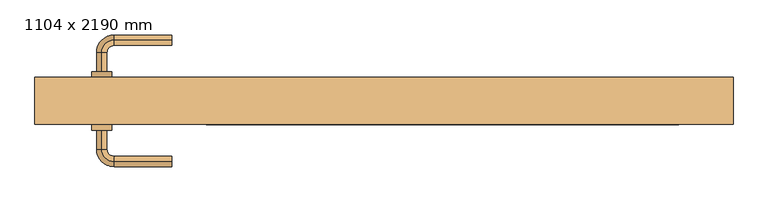
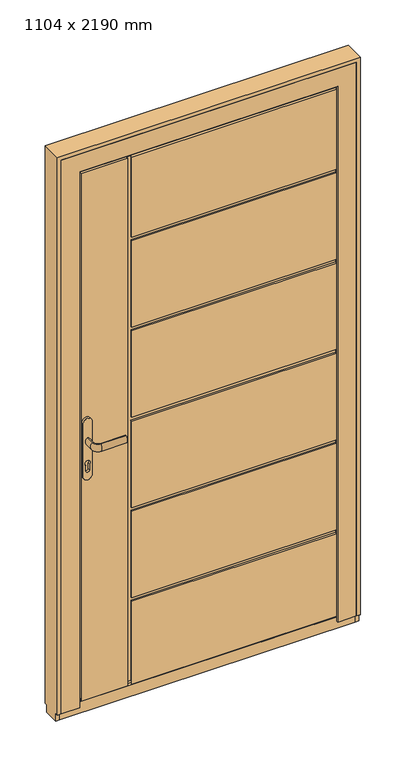
"""IFC4 building model written with IfcOpenShell, lengths in millimetres: door geometry, 1104 x 2190 mm."""

from ifc_helpers import new_model, si_unit, point, frame, frame_2d, origin, place, context, project, spatial, polyline, circle_curve, ellipse_curve, trimmed, segment, composite_curve, outline, extrude, faceted_brep, source, transform, mapped, element, save
from ifc_brep_helpers import plane_surface, revolved_surface, extruded_surface, advanced_brep


def door_1104_x_2190_mm_38c8fb91(model_context):
    return source(origin(), model_context, "Body", "SolidModel", [
        advanced_brep(
        [(-458.7, 104.0, 1064.0), (-458.7, 104.0, 1036.0), (-345.2, 155.0, 1064.0), (-345.2, 155.0, 1036.0), (-458.7, 135.0, 1036.0), (-458.7, 135.0, 1064.0), (-438.7, 155.0, 1036.0), (-438.7, 155.0, 1064.0)],
        [
            (0, 1, ellipse_curve(frame((-458.7, 104.0, 1050.0), z_axis=(0.0, -1.0, 0.0), x_axis=(0.0, 0.0, -1.0)), 14.0, 8.5)),
            (1, 0, ellipse_curve(frame((-458.7, 104.0, 1050.0), z_axis=(0.0, -1.0, 0.0), x_axis=(0.0, 0.0, -1.0)), 14.0, 8.5)),
            (2, 3, ellipse_curve(frame((-345.2, 155.0, 1050.0), z_axis=(1.0, 0.0, 0.0), x_axis=(0.0, 0.0, -1.0)), 14.0, 8.5)),
            (3, 2, ellipse_curve(frame((-345.2, 155.0, 1050.0), z_axis=(1.0, 0.0, 0.0), x_axis=(0.0, 0.0, -1.0)), 14.0, 8.5)),
            (1, 4),
            (4, 5, ellipse_curve(frame((-458.7, 135.0, 1050.0), z_axis=(0.0, -1.0, 0.0), x_axis=(0.0, 0.0, -1.0)), 14.0, 8.5)),
            (5, 0),
            (5, 4, ellipse_curve(frame((-458.7, 135.0, 1050.0), z_axis=(0.0, -1.0, 0.0), x_axis=(0.0, 0.0, -1.0)), 14.0, 8.5)),
            (6, 3),
            (2, 7),
            (7, 6, ellipse_curve(frame((-438.7, 155.0, 1050.0), z_axis=(1.0, 0.0, 0.0), x_axis=(0.0, 0.0, -1.0)), 14.0, 8.5)),
            (6, 7, ellipse_curve(frame((-438.7, 155.0, 1050.0), z_axis=(1.0, 0.0, 0.0), x_axis=(0.0, 0.0, -1.0)), 14.0, 8.5)),
            (7, 5, circle_curve(frame((-438.7, 135.0, 1064.0), z_axis=(0.0, 0.0, 1.0), x_axis=(-1.0, 0.0, 0.0)), 20.0)),
            (4, 6, circle_curve(frame((-438.7, 135.0, 1036.0), z_axis=(0.0, 0.0, -1.0), x_axis=(-1.0, 0.0, 0.0)), 20.0)),
        ],
        [
            plane_surface(frame((-458.7, 104.0, 1050.0), z_axis=(0.0, -1.0, 0.0), x_axis=(0.0, 0.0, 1.0))),
            plane_surface(frame((-345.2, 155.0, 1050.0), z_axis=(1.0, 0.0, 0.0), x_axis=(0.0, 0.0, 1.0))),
            extruded_surface(trimmed(ellipse_curve(frame((-458.7, 104.0, 1050.0), z_axis=(0.0, 1.0, 0.0), x_axis=(0.0, 0.0, -1.0)), 14.0, 8.5), [point((-458.7, 104.0, 1064.0))], [point((-458.7, 104.0, 1036.0))], True, "CARTESIAN"), (0.0, 31.0, 0.0), 31.0),
            extruded_surface(trimmed(ellipse_curve(frame((-458.7, 104.0, 1050.0), z_axis=(0.0, 1.0, 0.0), x_axis=(0.0, 0.0, -1.0)), 14.0, 8.5), [point((-458.7, 104.0, 1036.0))], [point((-458.7, 104.0, 1064.0))], True, "CARTESIAN"), (0.0, 31.0, 0.0), 31.0),
            extruded_surface(trimmed(ellipse_curve(frame((-438.7, 155.0, 1050.0), z_axis=(1.0, 0.0, 0.0), x_axis=(0.0, 0.0, -1.0)), 14.0, 8.5), [point((-438.7, 155.0, 1064.0))], [point((-438.7, 155.0, 1036.0))], True, "CARTESIAN"), (93.5, 0.0, 0.0), 93.5),
            extruded_surface(trimmed(ellipse_curve(frame((-438.7, 155.0, 1050.0), z_axis=(1.0, 0.0, 0.0), x_axis=(0.0, 0.0, -1.0)), 14.0, 8.5), [point((-438.7, 155.0, 1036.0))], [point((-438.7, 155.0, 1064.0))], True, "CARTESIAN"), (93.5, 0.0, 0.0), 93.5),
            revolved_surface(trimmed(ellipse_curve(frame((-458.7, 135.0, 1050.0), z_axis=(0.0, 1.0, 0.0), x_axis=(0.0, 0.0, -1.0)), 14.0, 8.5), [point((-458.7, 135.0, 1064.0))], [point((-458.7, 135.0, 1036.0))], True, "CARTESIAN"), (-438.7, 135.0, 1050.0), (0.0, 0.0, 1.0)),
            revolved_surface(trimmed(ellipse_curve(frame((-458.7, 135.0, 1050.0), z_axis=(0.0, 1.0, 0.0), x_axis=(0.0, 0.0, -1.0)), 14.0, 8.5), [point((-458.7, 135.0, 1036.0))], [point((-458.7, 135.0, 1064.0))], True, "CARTESIAN"), (-438.7, 135.0, 1050.0), (0.0, 0.0, 1.0)),
        ],
        [
            (0, [[1, 2]]),
            (1, [[3, 4]]),
            (2, [[5, 6, 7, -2]]),
            (3, [[-7, 8, -5, -1]]),
            (4, [[9, -3, 10, 11]]),
            (5, [[-10, -4, -9, 12]]),
            (6, [[-11, 13, -6, 14]]),
            (7, [[-12, -14, -8, -13]]),
        ],
    ),
        extrude(outline(composite_curve([segment(polyline([(1124.5, -475.2), (914.5, -475.2)]), True, "CONTINUOUS"), segment(trimmed(circle_curve(frame_2d((914.5, -458.7)), 16.5), [point((914.5, -475.2))], [point((914.5, -442.2))], False, "CARTESIAN"), True, "CONTINUOUS"), segment(polyline([(914.5, -442.2), (1124.5, -442.2)]), True, "CONTINUOUS"), segment(trimmed(circle_curve(frame_2d((1124.5, -458.7)), 16.5), [point((1124.5, -442.2))], [point((1124.5, -475.2))], False, "CARTESIAN"), True, "CONTINUOUS")], self_intersect=False), holes=[composite_curve([segment(trimmed(circle_curve(frame_2d((963.5537881, -458.7)), 10.0), [point((956.4123597, -465.7))], [point((956.4123597, -451.7))], True, "CARTESIAN"), True, "CONTINUOUS"), segment(polyline([(956.4123597, -451.7), (935.5537881, -451.7)]), True, "CONTINUOUS"), segment(trimmed(circle_curve(frame_2d((935.5537881, -458.7)), 7.0), [point((935.5537881, -451.7))], [point((935.5537881, -465.7))], True, "CARTESIAN"), True, "CONTINUOUS"), segment(polyline([(935.5537881, -465.7), (956.4123597, -465.7)]), True, "CONTINUOUS")], self_intersect=False)]), frame((0.0, 95.0, 0.0), z_axis=(0.0, 1.0, 0.0), x_axis=(0.0, 0.0, 1.0)), (0.0, 0.0, 1.0), 9.0),
        advanced_brep(
        [(-458.7, 9.0, 1064.0), (-458.7, 9.0, 1036.0), (-345.2, -42.0, 1064.0), (-345.2, -42.0, 1036.0), (-458.7, -22.0, 1064.0), (-458.7, -22.0, 1036.0), (-438.7, -42.0, 1036.0), (-438.7, -42.0, 1064.0)],
        [
            (0, 1, ellipse_curve(frame((-458.7, 9.0, 1050.0), z_axis=(0.0, 1.0, 0.0), x_axis=(0.0, 0.0, -1.0)), 14.0, 8.5)),
            (1, 0, ellipse_curve(frame((-458.7, 9.0, 1050.0), z_axis=(0.0, 1.0, 0.0), x_axis=(0.0, 0.0, -1.0)), 14.0, 8.5)),
            (2, 3, ellipse_curve(frame((-345.2, -42.0, 1050.0), z_axis=(1.0, 0.0, 0.0), x_axis=(0.0, 0.0, -1.0)), 14.0, 8.5)),
            (3, 2, ellipse_curve(frame((-345.2, -42.0, 1050.0), z_axis=(1.0, 0.0, 0.0), x_axis=(0.0, 0.0, -1.0)), 14.0, 8.5)),
            (0, 4),
            (4, 5, ellipse_curve(frame((-458.7, -22.0, 1050.0), z_axis=(0.0, 1.0, 0.0), x_axis=(0.0, 0.0, -1.0)), 14.0, 8.5)),
            (5, 1),
            (5, 4, ellipse_curve(frame((-458.7, -22.0, 1050.0), z_axis=(0.0, 1.0, 0.0), x_axis=(0.0, 0.0, -1.0)), 14.0, 8.5)),
            (6, 7, ellipse_curve(frame((-438.7, -42.0, 1050.0), z_axis=(1.0, 0.0, 0.0), x_axis=(0.0, 0.0, -1.0)), 14.0, 8.5)),
            (7, 2),
            (3, 6),
            (7, 6, ellipse_curve(frame((-438.7, -42.0, 1050.0), z_axis=(1.0, 0.0, 0.0), x_axis=(0.0, 0.0, -1.0)), 14.0, 8.5)),
            (6, 5, circle_curve(frame((-438.7, -22.0, 1036.0), z_axis=(0.0, 0.0, -1.0), x_axis=(-1.0, 0.0, 0.0)), 20.0)),
            (4, 7, circle_curve(frame((-438.7, -22.0, 1064.0), z_axis=(0.0, 0.0, 1.0), x_axis=(-1.0, 0.0, 0.0)), 20.0)),
        ],
        [
            plane_surface(frame((-458.7, 9.0, 1050.0), z_axis=(0.0, 1.0, 0.0), x_axis=(0.0, 0.0, 1.0))),
            plane_surface(frame((-345.2, -42.0, 1050.0), z_axis=(1.0, 0.0, 0.0), x_axis=(0.0, 0.0, 1.0))),
            extruded_surface(trimmed(ellipse_curve(frame((-458.7, -22.0, 1050.0), z_axis=(0.0, 1.0, 0.0), x_axis=(0.0, 0.0, -1.0)), 14.0, 8.5), [point((-458.7, -22.0, 1064.0))], [point((-458.7, -22.0, 1036.0))], True, "CARTESIAN"), (0.0, 31.0, 0.0), 31.0),
            extruded_surface(trimmed(ellipse_curve(frame((-458.7, -22.0, 1050.0), z_axis=(0.0, 1.0, 0.0), x_axis=(0.0, 0.0, -1.0)), 14.0, 8.5), [point((-458.7, -22.0, 1036.0))], [point((-458.7, -22.0, 1064.0))], True, "CARTESIAN"), (0.0, 31.0, 0.0), 31.0),
            extruded_surface(trimmed(ellipse_curve(frame((-345.2, -42.0, 1050.0), z_axis=(-1.0, 0.0, 0.0), x_axis=(0.0, 0.0, -1.0)), 14.0, 8.5), [point((-345.2, -42.0, 1064.0))], [point((-345.2, -42.0, 1036.0))], True, "CARTESIAN"), (-93.5, 0.0, 0.0), 93.5),
            extruded_surface(trimmed(ellipse_curve(frame((-345.2, -42.0, 1050.0), z_axis=(-1.0, 0.0, 0.0), x_axis=(0.0, 0.0, -1.0)), 14.0, 8.5), [point((-345.2, -42.0, 1036.0))], [point((-345.2, -42.0, 1064.0))], True, "CARTESIAN"), (-93.5, 0.0, 0.0), 93.5),
            revolved_surface(trimmed(ellipse_curve(frame((-458.7, -22.0, 1050.0), z_axis=(0.0, 1.0, 0.0), x_axis=(0.0, 0.0, -1.0)), 14.0, 8.5), [point((-458.7, -22.0, 1064.0))], [point((-458.7, -22.0, 1036.0))], True, "CARTESIAN"), (-438.7, -22.0, 1050.0), (0.0, 0.0, 1.0)),
            revolved_surface(trimmed(ellipse_curve(frame((-458.7, -22.0, 1050.0), z_axis=(0.0, 1.0, 0.0), x_axis=(0.0, 0.0, -1.0)), 14.0, 8.5), [point((-458.7, -22.0, 1036.0))], [point((-458.7, -22.0, 1064.0))], True, "CARTESIAN"), (-438.7, -22.0, 1050.0), (0.0, 0.0, 1.0)),
        ],
        [
            (0, [[1, 2]]),
            (1, [[3, 4]]),
            (2, [[-1, 5, 6, 7]]),
            (3, [[-2, -7, 8, -5]]),
            (4, [[9, 10, -4, 11]]),
            (5, [[12, -11, -3, -10]]),
            (6, [[13, -6, 14, -9]]),
            (7, [[-14, -8, -13, -12]]),
        ],
    ),
        extrude(outline(composite_curve([segment(polyline([(1124.5, -475.2), (914.5, -475.2)]), True, "CONTINUOUS"), segment(trimmed(circle_curve(frame_2d((914.5, -458.7)), 16.5), [point((914.5, -475.2))], [point((914.5, -442.2))], False, "CARTESIAN"), True, "CONTINUOUS"), segment(polyline([(914.5, -442.2), (1124.5, -442.2)]), True, "CONTINUOUS"), segment(trimmed(circle_curve(frame_2d((1124.5, -458.7)), 16.5), [point((1124.5, -442.2))], [point((1124.5, -475.2))], False, "CARTESIAN"), True, "CONTINUOUS")], self_intersect=False), holes=[composite_curve([segment(trimmed(circle_curve(frame_2d((963.5537881, -458.7)), 10.0), [point((956.4123597, -465.7))], [point((956.4123597, -451.7))], True, "CARTESIAN"), True, "CONTINUOUS"), segment(polyline([(956.4123597, -451.7), (935.5537881, -451.7)]), True, "CONTINUOUS"), segment(trimmed(circle_curve(frame_2d((935.5537881, -458.7)), 7.0), [point((935.5537881, -451.7))], [point((935.5537881, -465.7))], True, "CARTESIAN"), True, "CONTINUOUS"), segment(polyline([(935.5537881, -465.7), (956.4123597, -465.7)]), True, "CONTINUOUS")], self_intersect=False)]), frame((0.0, 9.0, 0.0), z_axis=(0.0, 1.0, 0.0), x_axis=(0.0, 0.0, 1.0)), (0.0, 0.0, 1.0), 9.0),
        faceted_brep([(-288.7, 25.0, 366.5833337), (-288.7, 25.0, 708.166667), (478.7, 25.0, 708.166667), (478.7, 25.0, 723.166667), (-288.7, 25.0, 723.166667), (-288.7, 25.0, 1064.7500004), (478.7, 25.0, 1064.7500004), (478.7, 25.0, 1079.7500004), (-288.7, 25.0, 1079.7500004), (-288.7, 25.0, 1421.3333337), (478.7, 25.0, 1421.3333337), (478.7, 25.0, 1436.3333337), (-288.7, 25.0, 1436.3333337), (-288.7, 25.0, 1777.916667), (478.7, 25.0, 1777.916667), (478.7, 25.0, 1792.916667), (-288.7, 25.0, 1792.916667), (-288.7, 25.0, 2109.5000003), (-303.7, 25.0, 2109.5000003), (-303.7, 25.0, 35.0), (-288.7, 25.0, 35.0), (-288.7, 25.0, 351.5833337), (478.7, 25.0, 351.5833337), (478.7, 25.0, 366.5833337), (-288.7, 18.0, 366.5833337), (-288.7, 18.0, 708.166667), (478.7, 18.0, 708.166667), (478.7, 27.0002302, 2109.5000003), (478.7, 18.0, 2109.5000003), (478.7, 18.0, 1792.916667), (478.7, 18.0, 1777.916667), (478.7, 18.0, 1436.3333337), (478.7, 18.0, 1421.3333337), (478.7, 18.0, 1079.7500004), (478.7, 18.0, 1064.7500004), (478.7, 18.0, 723.166667), (478.7, 18.0, 366.5833337), (478.7, 18.0, 351.5833337), (478.7, 18.0, 24.0), (478.7, 19.9979528, 24.0), (478.7, 19.9979528, 35.0), (478.7, 27.0002302, 35.0), (-288.7, 18.0, 723.166667), (-288.7, 18.0, 1064.7500004), (-288.7, 18.0, 1079.7500004), (-288.7, 18.0, 1421.3333337), (-303.7, 18.0, 2109.5000003), (-303.7, 18.0, 24.0), (-303.7, 19.9979528, 24.0), (-303.7, 19.9979528, 35.0), (-288.7, 19.9979528, 35.0), (-478.7, 19.9979528, 35.0), (-478.7, 27.0002302, 35.0), (-288.7, 18.0, 351.5833337), (-288.7, 19.9979528, 24.0), (-288.7, 18.0, 24.0), (-478.7, 19.9979528, 24.0), (-478.7, 18.0, 24.0), (-478.7, 18.0, 2109.5000003), (-288.7, 18.0, 1777.916667), (-288.7, 18.0, 1436.3333337), (-288.7, 18.0, 2109.5000003), (-288.7, 18.0, 1792.916667), (503.7, 95.0, 10.0000003), (503.7, 92.0, 10.0000003), (-288.7, 92.0, 10.0000003), (-288.7, 95.0, 10.0000003), (-503.7, 92.0, 10.0000003), (-503.7, 95.0, 10.0000003), (-303.7, 95.0, 10.0000003), (-303.7, 92.0, 10.0000003), (503.7, 95.0, 351.5833337), (503.7, 92.0, 351.5833337), (503.7, 95.0, 366.5833337), (503.7, 95.0, 708.166667), (503.7, 92.0, 708.166667), (503.7, 92.0, 366.5833337), (503.7, 95.0, 1079.7500004), (503.7, 95.0, 1421.3333337), (503.7, 92.0, 1421.3333337), (503.7, 92.0, 1079.7500004), (503.7, 95.0, 723.166667), (503.7, 95.0, 1064.7500004), (503.7, 92.0, 1064.7500004), (503.7, 92.0, 723.166667), (503.7, 95.0, 1436.3333337), (503.7, 95.0, 1777.916667), (503.7, 92.0, 1777.916667), (503.7, 92.0, 1436.3333337), (503.7, 95.0, 2134.5000003), (503.7, 92.0, 2134.5000003), (503.7, 92.0, 1792.916667), (503.7, 95.0, 1792.916667), (488.2, 92.0, 351.5833337), (488.2, 92.0, 25.5), (-288.7, 92.0, 25.5), (488.2, 92.0, 708.166667), (488.2, 92.0, 366.5833337), (488.2, 92.0, 1421.3333337), (488.2, 92.0, 1079.7500004), (488.2, 92.0, 1064.7500004), (488.2, 92.0, 723.166667), (488.2, 92.0, 1777.916667), (488.2, 92.0, 1436.3333337), (-288.7, 92.0, 2134.5000003), (-288.7, 92.0, 2119.0000003), (488.2, 92.0, 2119.0000003), (488.2, 92.0, 1792.916667), (-488.2, 92.0, 25.5), (-488.2, 92.0, 2119.0000003), (-303.7, 92.0, 2119.0000003), (-303.7, 92.0, 2134.5000003), (-503.7, 92.0, 2134.5000003), (-303.7, 92.0, 25.5), (-288.7, 88.0, 351.5833337), (-288.7, 95.0, 351.5833337), (-288.7, 88.0, 25.5), (-288.7, 95.0, 366.5833337), (-288.7, 95.0, 708.166667), (-288.7, 95.0, 1079.7500004), (-288.7, 95.0, 1421.3333337), (-288.7, 95.0, 723.166667), (-288.7, 95.0, 1064.7500004), (-288.7, 95.0, 1436.3333337), (-288.7, 95.0, 1777.916667), (-288.7, 95.0, 1792.916667), (-288.7, 95.0, 2134.5000003), (-503.7, 95.0, 2134.5000003), (-303.7, 95.0, 2134.5000003), (-303.7, 88.0, 2119.0000003), (-303.7, 88.0, 25.5), (-478.7, 27.0002302, 2109.5000003), (488.2, 27.0002302, 2119.0000003), (-488.2, 27.0002302, 2119.0000003), (-488.2, 27.0002302, 25.5), (488.2, 27.0002302, 25.5), (488.2, 88.0, 351.5833337), (488.2, 88.0, 366.5833337), (488.2, 88.0, 708.166667), (488.2, 88.0, 723.166667), (488.2, 88.0, 1064.7500004), (488.2, 88.0, 1079.7500004), (488.2, 88.0, 1421.3333337), (488.2, 88.0, 1436.3333337), (488.2, 88.0, 1777.916667), (488.2, 88.0, 1792.916667), (-288.7, 88.0, 1777.916667), (-288.7, 88.0, 1436.3333337), (-288.7, 88.0, 1421.3333337), (-288.7, 88.0, 1079.7500004), (-288.7, 88.0, 1064.7500004), (-288.7, 88.0, 723.166667), (-288.7, 88.0, 708.166667), (-288.7, 88.0, 366.5833337), (-288.7, 88.0, 2119.0000003), (-288.7, 88.0, 1792.916667)], [[[0, 1, 2, 3, 4, 5, 6, 7, 8, 9, 10, 11, 12, 13, 14, 15, 16, 17, 18, 19, 20, 21, 22, 23]], [[1, 0, 24, 25]], [[1, 25, 26, 2]], [[27, 28, 29, 15, 14, 30, 31, 11, 10, 32, 33, 7, 6, 34, 35, 3, 2, 26, 36, 23, 22, 37, 38, 39, 40, 41]], [[42, 4, 3, 35]], [[5, 4, 42, 43]], [[5, 43, 34, 6]], [[44, 8, 7, 33]], [[9, 8, 44, 45]], [[19, 18, 46, 47, 48, 49]], [[41, 40, 50, 20, 19, 49, 51, 52]], [[53, 21, 20, 50, 54, 55]], [[21, 53, 37, 22]], [[24, 0, 23, 36]], [[40, 39, 54, 50]], [[56, 51, 49, 48]], [[39, 38, 55, 54]], [[57, 56, 48, 47]], [[33, 32, 45, 44]], [[35, 34, 43, 42]], [[36, 26, 25, 24]], [[55, 38, 37, 53]], [[58, 57, 47, 46]], [[31, 30, 59, 60]], [[28, 61, 62, 29]], [[63, 64, 65, 66]], [[67, 68, 69, 70]], [[64, 63, 71, 72]], [[73, 74, 75, 76]], [[77, 78, 79, 80]], [[81, 82, 83, 84]], [[85, 86, 87, 88]], [[89, 90, 91, 92]], [[65, 64, 72, 93, 94, 95]], [[76, 75, 96, 97]], [[80, 79, 98, 99]], [[84, 83, 100, 101]], [[88, 87, 102, 103]], [[90, 104, 105, 106, 107, 91]], [[108, 109, 110, 111, 112, 67, 70, 113]], [[114, 115, 66, 65, 95, 116]], [[63, 66, 115, 71]], [[74, 73, 117, 118]], [[78, 77, 119, 120]], [[82, 81, 121, 122]], [[86, 85, 123, 124]], [[89, 92, 125, 126]], [[68, 127, 128, 69]], [[68, 67, 112, 127]], [[129, 130, 113, 70, 69, 128, 111, 110]], [[58, 131, 52, 51, 56, 57]], [[132, 133, 134, 135], [131, 27, 41, 52]], [[106, 132, 135, 94, 93, 136, 137, 97, 96, 138, 139, 101, 100, 140, 141, 99, 98, 142, 143, 103, 102, 144, 145, 107]], [[94, 135, 134, 108, 113, 130, 116, 95]], [[133, 109, 108, 134]], [[146, 147, 143, 142, 148, 149, 141, 140, 150, 151, 139, 138, 152, 153, 137, 136, 114, 116, 130, 129, 154, 155, 145, 144]], [[149, 148, 120, 119]], [[149, 119, 77, 80, 99, 141]], [[122, 150, 140, 100, 83, 82]], [[151, 150, 122, 121]], [[151, 121, 81, 84, 101, 139]], [[118, 152, 138, 96, 75, 74]], [[153, 152, 118, 117]], [[153, 117, 73, 76, 97, 137]], [[115, 114, 136, 93, 72, 71]], [[9, 45, 32, 10]], [[60, 12, 11, 31]], [[13, 12, 60, 59]], [[13, 59, 30, 14]], [[62, 16, 15, 29]], [[16, 62, 61, 17]], [[124, 146, 144, 102, 87, 86]], [[125, 155, 154, 105, 104, 126]], [[120, 148, 142, 98, 79, 78]], [[147, 123, 85, 88, 103, 143]], [[147, 146, 124, 123]], [[155, 125, 92, 91, 107, 145]], [[90, 89, 126, 104]], [[127, 112, 111, 128]], [[132, 106, 105, 154, 129, 110, 109, 133]], [[27, 131, 58, 46, 18, 17, 61, 28]]]),
        faceted_brep([(-552.25, 95.0, 0.0), (-507.75, 95.0, 0.0), (-507.75, 86.0, 0.0), (-552.25, 85.9997571, 0.0), (-498.25, 22.5000042, 0.0), (-482.75, 22.5000042, 0.0), (-482.75, 18.0, 0.0), (-552.25, 18.0, 0.0), (-552.25, 27.0, 0.0), (-498.25, 27.0, 0.0), (552.25, 18.0, 0.0), (482.75, 18.0, 0.0), (482.75, 22.5000042, 0.0), (498.25, 22.5000042, 0.0), (498.25, 27.0, 0.0), (552.25, 27.0, 0.0), (507.75, 86.0, 0.0), (507.75, 95.0, 0.0), (552.25, 95.0, 0.0), (552.25, 85.9997571, 0.0), (-552.25, 18.0, 2189.5), (-552.25, 95.0, 2189.5), (-552.25, 85.9997571, -30.0), (-552.25, 27.0, -30.0), (552.25, 95.0, 2189.5), (507.75, 95.0, 2145.0), (-507.75, 95.0, 2145.0), (552.25, 18.0, 2189.5), (552.25, 27.0, -30.0), (552.25, 85.9997571, -30.0), (-482.75, 18.0, 2120.0), (482.75, 18.0, 2120.0), (-498.25, 86.0, 2135.5), (-498.25, 22.5000042, 2135.5), (-498.25, 27.0, 14.5), (-498.25, 86.0, 14.5), (498.25, 86.0, 2135.5), (498.25, 22.5000042, 2135.5), (498.25, 86.0, 14.5), (498.25, 27.0, 14.5), (-507.75, 86.0, 2145.0), (507.75, 86.0, 2145.0), (482.75, 22.5000042, 2120.0), (-482.75, 22.5000042, 2120.0)], [[[0, 1, 2, 3]], [[4, 5, 6, 7, 8, 9]], [[10, 11, 12, 13, 14, 15]], [[16, 17, 18, 19]], [[7, 20, 21, 0, 3, 22, 23, 8]], [[1, 0, 21, 24, 18, 17, 25, 26]], [[21, 20, 27, 24]], [[18, 24, 27, 10, 15, 28, 29, 19]], [[7, 6, 30, 31, 11, 10, 27, 20]], [[32, 33, 4, 9, 34, 35]], [[33, 32, 36, 37]], [[37, 36, 38, 39, 14, 13]], [[40, 2, 1, 26]], [[16, 19, 29, 22, 3, 2, 40, 41], [36, 32, 35, 38]], [[5, 4, 33, 37, 13, 12, 42, 43]], [[6, 5, 43, 30]], [[26, 25, 41, 40]], [[31, 30, 43, 42]], [[17, 16, 41, 25]], [[12, 11, 31, 42]], [[23, 28, 15, 14, 39, 34, 9, 8]], [[38, 35, 34, 39]], [[23, 22, 29, 28]]]),
        faceted_brep([(-552.25, 86.0, -30.0), (-552.25, 27.0, -30.0), (-567.25, 27.0, -30.0), (-567.25, 86.0, -30.0), (-552.25, 95.0, 2189.5), (-552.25, 18.0, 2189.5), (-552.25, 18.0, 0.0), (-552.25, 27.0, 0.0), (-552.25, 86.0, 0.0), (-552.25, 95.0, 0.0), (567.25, 27.0, 0.0), (552.25, 27.0, 0.0), (552.25, 27.0, -30.0), (567.25, 27.0, -30.0), (-567.25, 27.0, 0.0), (-567.25, 18.0, 2204.5), (-567.25, 95.0, 2204.5), (-567.25, 95.0, 0.0), (-567.25, 86.0, 0.0), (-567.25, 18.0, 0.0), (552.25, 86.0, 0.0), (567.25, 86.0, 0.0), (567.25, 86.0, -30.0), (552.25, 86.0, -30.0), (552.25, 18.0, 2189.5), (552.25, 95.0, 2189.5), (552.25, 95.0, 0.0), (552.25, 18.0, 0.0), (567.25, 95.0, 2204.5), (567.25, 95.0, 0.0), (567.25, 18.0, 0.0), (567.25, 18.0, 2204.5)], [[[0, 1, 2, 3]], [[4, 5, 6, 7, 1, 0, 8, 9]], [[10, 11, 12, 13]], [[7, 14, 2, 1]], [[15, 16, 17, 18, 3, 2, 14, 19]], [[20, 21, 22, 23]], [[18, 8, 0, 3]], [[24, 25, 26, 20, 23, 12, 11, 27]], [[25, 4, 9, 17, 16, 28, 29, 26]], [[21, 20, 26, 29]], [[8, 18, 17, 9]], [[22, 13, 12, 23]], [[11, 10, 30, 27]], [[14, 7, 6, 19]], [[5, 24, 27, 30, 31, 15, 19, 6]], [[28, 31, 30, 10, 13, 22, 21, 29]], [[5, 4, 25, 24]], [[16, 15, 31, 28]]]),
    ])


if __name__ == "__main__":
    model = new_model("IFC4")
    model_context = context("Model", 3, world=origin())
    ifc_project = project(units=[si_unit("LENGTHUNIT", "METRE", prefix="MILLI")], contexts=[model_context])
    site = spatial("IfcSite", under=ifc_project)
    building = spatial("IfcBuilding", under=site)
    placement = place(None, origin())
    door_1104_x_2190_mm_shape = door_1104_x_2190_mm_38c8fb91(model_context)
    element("IfcDoor", 1, ObjectType="1104 x 2190 mm", at=placement, inside=building, context=model_context, shape_type="MappedRepresentation", body=[
        mapped(door_1104_x_2190_mm_shape, transform((0.0, 0.0, 0.0), x_axis=(1.0, 0.0, 0.0), y_axis=(0.0, 1.0, 0.0), z_axis=(0.0, 0.0, 1.0))),
    ])
    save(model, "model.ifc")

# Revit data of these elements
# Type "1104 x 2190 mm"
#   Type Mark = "28"
#   Water resistance = "up to Class E900, EN 12208:2001"
#   Uniclass2015Version = "v1.21"
#   Uniclass2015Reference = "Ss_25_30_20_30"
#   Uniclass2015Description = "Frame and door leaf system"
#   URL = "www.aluprof.eu"
#   Type IFC Predefined Type = "USERDEFINED"
#   Right-hand / Left-hand door [instance default] = ""
#   Resistance to wind load = "up to Class C5/B5, EN 12210:2001"
#   Insert type = "ST"
#   Hardware [instance default] = ""
#   Product page = "https://aluprof.eu/en/architects/offer/window-and-door-systems/panel-doors#visualisation"
#   Operation = "SinglePanelOutwardOpening"
#   Opening type = "Outward"
#   NBSReference = "25-50-20/125"
#   NBSDescription = "Frame and door leaf system"
#   Important = "The actual acceptable construction dimensions are dependent on the selection of profiles and hardware, glazing type, construction weight and the construction’s operating conditions. These should be determined by a suitably qualified person, and using ALUPROF’s calculation software"
#   IfcExportType = "USERDEFINED"
#   IfcExportAs = "IfcDoorType"
#   Handle type [instance default] = ""
#   Manufacturer = "ALUPROF"
#   Export Type to IFC As = "IfcDoorType"
#   Door sill type [instance default] = ""
#   Description = "External single-leaf panel door outward opening"
#   Model = "MB-86 ST Panel Door AD07"
#   Content of the recyclate in the material = "69.2"
#   COBie.Type.WarrantyDurationParts = ""
#   COBie.Type.Name = ""
#   COBie.Type.Manufacturer = "ALUPROF S.A."
#   COBie.Space.Name = ""
#   COBie.Floor.Name = ""
#   COBie.Facility.Name = ""
#   COBie.CreatedOn = ""
#   COBie.Component.WarrantyStartDate = ""
#   COBie.Component.Name = "MB-86 ST Panel Door AD07"
#   Burglar resistance = "RC2"
#   Air permeability = "up to Class 4, EN 12207:2001"
#   Width of the active leaf = 1007.4 mm
#   Placement in wall = 20 mm
#   Thickness = 77 mm
#   Height of the opening sash = 2124.5 mm
#   Handle Offset = 1050 mm
#   Glazing thickness = 48 mm
#   Rough Height = 2250.7 mm
#   Rough Width = 1134.5 mm
#   Height = 2189.5 mm
#   Width = 1104.5 mm
#   Construction depth = 77 mm
#   Clear opening width = 900 mm
#   Clear opening height = 2100 mm
#   Height of the array = 341.583 mm
#   Schedule No. [instance default] = 1
#   Handrail = no
#   IsExternal = yes
#   Handle = yes
#   Door closer [instance default] = no
#   Function = 1
#   COBie.Type = yes
#   COBie = yes
#   Access control [instance default] = no
#   Panel = element 260956
#   Wall Closure = (empty or 0)
